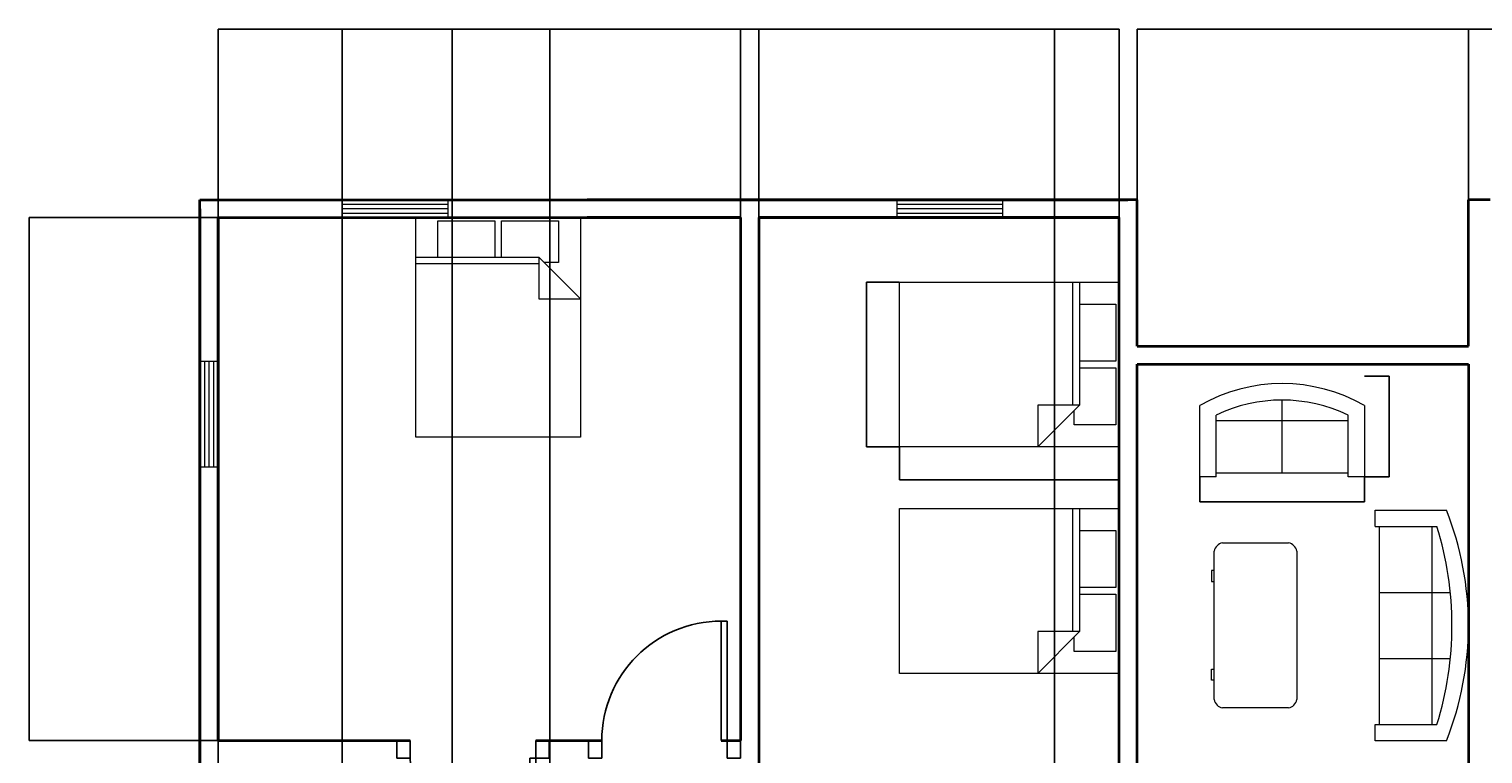
# Model space of a CAD drawing. Units: millimetres. Extents: x 31 to 27050, y -916 to 32407.
# Tile 6 of 7: x 31 to 13474, y 25704 to 32407. Entities that reach past the tile are written whole.
import ezdxf

# ---------------------------------------------------------------- set-up
doc = ezdxf.new("R2010")
doc.units = ezdxf.units.MM
for name, color, linetype, lineweight in [('A-ANNO-DIMS', 2, 'Continuous', 18), ('A-DOOR', 3, 'Continuous', 25), ('A-FURN', 8, 'Continuous', 13), ('A-GLAZ', 4, 'Continuous', 18), ('A-WALL', 7, 'Continuous', 35)]:
    doc.layers.add(name, color=color, linetype=linetype, lineweight=lineweight)
doc.styles.get("Standard").update_dxf_attribs({"font": 'arial.ttf'})
doc.dimstyles.get("Standard").update_dxf_attribs({"dimtxt": 0.18, "dimasz": 0.18, "dimexe": 0.18, "dimexo": 0.0625, "dimgap": 0.09, "dimtad": 0, "dimtih": 1, "dimtoh": 1, "dimdec": 4, "dimzin": 0, "dimdsep": 46, "dimtxsty": 'Standard', "dimcen": 0.09, "dimadec": 0, "dimazin": 0, "dimtfac": 1, "dimtdec": 4, "dimtofl": 0, "dimtmove": 0, "dimatfit": 3, "dimfxl": 1, "dimtolj": 1, "dimtzin": 0, "dimarcsym": 0})

# ---------------------------------------------------------------- blocks, each defined once
blk = doc.blocks.new('Sofa - Roundback 7 ft.')
for p, q in [((-12.00002, -32.44210000000393), (-12.00003, -6.597100000003898)), ((11.99996999999999, -32.44210000000393), (11.99997999999999, -6.597100000003898)), ((-36.000027, -34.00000000000395), (-36.000027, -11.46960000000396)), ((-35.999844, -13.38190000000397), (35.99979999999999, -13.38190000000397)), ((35.99997999999999, -34.00000000000395), (35.99997999999999, -11.46960000000396)), ((-36.000027, -32.44210000000393), (35.99997999999999, -32.44210000000393))]:
    blk.add_line(p, q)
for points in [[(-36.000027, -34.00000000000395), (-42.000027, -34.00000000000395), (-42.000027, -8.000000000003944)], [(41.99997999999999, -8.000000000003944), (41.99997999999999, -34.00000000000395), (35.99997999999999, -34.00000000000395)]]:
    blk.add_lwpolyline(points)
for centre, radius, start, end in [((0, -114.2500000000039), 114.2500000000039, 68.43141000000072, 111.5686000000006), ((-1.00000000032e-05, -127.1968000000039), 121.1967999999973, 72.72032999999948, 107.2797000000005)]:
    blk.add_arc(centre, radius, start, end)
blk = doc.blocks.new('Sofa - Roundback Loveseat 5 ft.')
for p, q in [((0, -32.44198000000246), (0, -5.999980000002448)), ((-23.99999999999999, -33.99998000000245), (-23.99999999999999, -11.46958000000243)), ((-23.99979999999998, -13.38178000000245), (23.99986, -13.38178000000245)), ((24.00004000000001, -33.99998000000245), (24.00004000000001, -11.46958000000243)), ((-23.99999999999999, -32.44198000000246), (24.00004000000001, -32.44198000000246))]:
    blk.add_line(p, q)
for points in [[(-23.99999999999999, -33.99998000000245), (-29.99999999999999, -33.99998000000245), (-29.99999999999999, -7.999980000002448)], [(30.00004000000001, -7.999980000002448), (30.00004000000001, -33.99998000000245), (24.00004000000001, -33.99998000000245)]]:
    blk.add_lwpolyline(points)
for centre, radius, start, end in [((0, -60.24998000000245), 60.24998000000245, 60.13715000000122, 119.862800000004), ((0, -61.38438000000245), 55.38444000000723, 64.32083000000306, 115.6791999999996)]:
    blk.add_arc(centre, radius, start, end)
blk = doc.blocks.new('Desk - 30 x 60 in.')
for p, q in [((-26.999995, 0), (26.999995, 0)), ((-29.999995, -27), (-29.999995, -3)), ((29.999995, -3), (29.999995, -27)), ((26.999995, -30), (-26.999995, -30)), ((-20.000005, -30), (-20.000005, -31)), ((-20.000005, -31), (-16.000005, -31)), ((-16.000005, -31), (-16.000005, -30)), ((15.999995, -31), (15.999995, -30)), ((19.999995, -31), (15.999995, -31)), ((19.999995, -30), (19.999995, -31))]:
    blk.add_line(p, q)
for centre, radius, start, end in [((-26.499995, -3.5), 3.535534000004229, 98.1300999999916, 171.8698999999352), ((26.499995, -3.5), 3.535533999997753, 8.130102000022115, 81.8698999999439), ((-26.499995, -26.5), 3.535534000000845, 188.1301000000653, 261.8699000000085), ((26.499995, -26.5), 3.535534000004826, 278.1301000000561, 351.8698999999439)]:
    blk.add_arc(centre, radius, start, end)
blk = doc.blocks.new('Bed - Queen')
for p, q in [((0, -80.00003000000002), (0, 0)), ((0, 0), (59.99998999999999, 0)), ((59.99998999999999, 0), (59.99998999999999, -80.00003000000002)), ((7.99999, -1.200000000000017), (28.79998, -1.200000000000017)), ((7.99999, -14.4), (7.99999, -1.200000000000017)), ((28.79998, -1.200000000000017), (28.79998, -14.4)), ((31.19999, -1.200000000000017), (51.99999000000001, -1.200000000000017)), ((31.19999, -14.4), (31.19999, -1.200000000000017)), ((51.99999000000001, -1.200000000000017), (51.99999000000001, -16.4)), ((0, -14.4), (44.79999999999999, -14.4)), ((59.99998999999999, -29.60000000000001), (44.79999999999999, -14.4)), ((44.79999999999999, -14.4), (44.79999999999999, -29.60000000000001)), ((44.79999999999999, -16.80000000000001), (0, -16.80000000000001)), ((51.99999000000001, -16.4), (46.79936, -16.4)), ((44.79999999999999, -29.60000000000001), (59.99998999999999, -29.60000000000001)), ((59.99998999999999, -80.00003000000002), (0, -80.00003000000002))]:
    blk.add_line(p, q)
blk = doc.blocks.new('Window - Wood Frame 36 in. Wide plan')
for p, q in [((0, 6), (0, 0)), ((36, 6), (36, 0)), ((0, 4.5), (36, 4.5)), ((0, 3), (36, 3)), ((0, 1.5), (36, 1.5))]:
    blk.add_line(p, q)
blk = doc.blocks.new('DOOR-SINGLE-1104')
for p, q in [((56.41678681898429, 1104.337341461596), (-7.18501e-11, 1104.337341461596)), ((-7.18501e-11, 1104.337341461596), (-7.18501e-11, 3.638e-12)), ((56.41678681898429, 7.276e-12), (56.41678681898429, 1104.337341461596)), ((-1226.913698425656, -163.8831223050438), (-1226.913698425656, 3.638e-12)), ((-1104.337341461589, 3.638e-12), (-1226.913698425656, 7.276e-12)), ((-1104.337341461589, 3.638e-12), (-1104.337341461589, -163.8831223050438)), ((-7.18501e-11, 3.638e-12), (56.41678681898429, 7.276e-12)), ((56.41678681898429, -163.8831223050438), (56.41678681898429, 3.638e-12)), ((56.41678681898429, 3.638e-12), (178.9931437830519, 3.638e-12)), ((178.9931437830519, 3.638e-12), (178.9931437830519, -163.8831223050438)), ((-1104.337341461589, -163.8831223050438), (-1226.913698425656, -163.8831223050438)), ((178.9931437830519, -163.8831223050438), (56.41678681898429, -163.8831223050438))]:
    blk.add_line(p, q)
blk.add_arc((0, 3.638e-12), 1104.337341461589, 90, 180)
blk = doc.blocks.new('*D18')
at = {"layer": 'A-ANNO-DIMS', "color": 0, "lineweight": -2, "transparency": 16777216}
for p, q in [((8078.02123511446, 28542.79574648087), (8078.02123511446, 28237.87813218087)), ((10110.02199711446, 28542.79574648087), (10110.02199711446, 28237.87813218087)), ((8078.201235114461, 28238.05813218087), (9092.578362362754, 28238.05813218087)), ((10109.84199711446, 28238.05813218087), (9095.464869866166, 28238.05813218087))]:
    blk.add_line(p, q, dxfattribs=at)
at = {"layer": 'A-ANNO-DIMS', "color": 0, "transparency": 16777216}
for points in [[(8078.201235114461, 28238.08813218087), (8078.201235114461, 28238.02813218087), (8078.02123511446, 28238.05813218087)], [(10109.84199711446, 28238.08813218087), (10109.84199711446, 28238.02813218087), (10110.02199711446, 28238.05813218087)]]:
    blk.add_solid(points, dxfattribs=at)
at = {"layer": 'Defpoints', "color": 0, "transparency": 16777216}
for p in [(8078.02123511446, 28542.85824648087), (10110.02199711446, 28542.85824648087), (10110.02199711446, 28238.05813218087)]:
    blk.add_point(p, dxfattribs=at)
at = {"layer": 'A-ANNO-DIMS', "color": 0, "transparency": 16777216, "insert": (9094.02161611446, 28238.05813218087), "char_height": 0.18, "attachment_point": 5}
blk.add_mtext('\\A1;QUEEN BED 2032 TYP.', dxfattribs=at)
blk = doc.blocks.new('*D19')
at = {"layer": 'A-ANNO-DIMS', "color": 0, "lineweight": -2, "transparency": 16777216}
for p, q in [((8077.958735114462, 30066.85799248089), (7773.041120814466, 30066.85799248089)), ((7773.221120814466, 30066.67799248088), (7773.221120814466, 29305.04002261868)), ((7773.221120814466, 28543.03824648089), (7773.221120814466, 29304.6762163431)), ((8077.958735114462, 28542.85824648089), (7773.041120814466, 28542.85824648089))]:
    blk.add_line(p, q, dxfattribs=at)
at = {"layer": 'A-ANNO-DIMS', "color": 0, "transparency": 16777216}
for points in [[(7773.191120814466, 30066.67799248088), (7773.251120814466, 30066.67799248088), (7773.221120814466, 30066.85799248089)], [(7773.191120814466, 28543.03824648089), (7773.251120814466, 28543.03824648089), (7773.221120814466, 28542.85824648089)]]:
    blk.add_solid(points, dxfattribs=at)
at = {"layer": 'Defpoints', "color": 0, "transparency": 16777216}
for p in [(8078.021235114462, 30066.85799248089), (7773.221120814466, 28542.85824648089), (8078.021235114462, 28542.85824648089)]:
    blk.add_point(p, dxfattribs=at)
at = {"layer": 'A-ANNO-DIMS', "color": 0, "transparency": 16777216, "insert": (7773.221120814473, 29304.85811948088), "char_height": 0.18, "attachment_point": 5}
blk.add_mtext('\\A1;1524 TYP.', dxfattribs=at)
blk = doc.blocks.new('*D36')
at = {"layer": 'A-ANNO-DIMS', "color": 0, "lineweight": -2, "transparency": 16777216}
for p, q in [((10855.59232014758, 28264.73272793006), (10855.59232014758, 28036.01507553007)), ((12379.59333614758, 28264.73272793006), (12379.59333614758, 28036.01507553007)), ((10855.77232014758, 28036.19507553007), (11616.23012009846, 28036.19507553007)), ((12379.41333614758, 28036.19507553007), (11618.95553619669, 28036.19507553007))]:
    blk.add_line(p, q, dxfattribs=at)
at = {"layer": 'A-ANNO-DIMS', "color": 0, "transparency": 16777216}
for points in [[(10855.77232014758, 28036.22507553006), (10855.77232014758, 28036.16507553007), (10855.59232014758, 28036.19507553007)], [(12379.41333614758, 28036.22507553006), (12379.41333614758, 28036.16507553007), (12379.59333614758, 28036.19507553007)]]:
    blk.add_solid(points, dxfattribs=at)
at = {"layer": 'Defpoints', "color": 0, "transparency": 16777216}
for p in [(10855.59232014758, 28264.79522793006), (12379.59333614758, 28264.79522793006), (12379.59333614758, 28036.19507553007)]:
    blk.add_point(p, dxfattribs=at)
at = {"layer": 'A-ANNO-DIMS', "color": 0, "transparency": 16777216, "insert": (11617.59282814758, 28036.19507553007), "char_height": 0.18, "attachment_point": 5}
blk.add_mtext('\\A1;LOVESEAT 1524 TYP.', dxfattribs=at)
blk = doc.blocks.new('*D37')
at = {"layer": 'A-ANNO-DIMS', "color": 0, "lineweight": -2, "transparency": 16777216}
for p, q in [((12379.65583614758, 29196.12811589219), (12608.37348854759, 29196.12811589219)), ((12608.19348854759, 29195.94811589218), (12608.19348854759, 28730.64363644047)), ((12608.19348854759, 28264.97522793008), (12608.19348854759, 28730.2797073818)), ((12379.65583614758, 28264.79522793008), (12608.37348854759, 28264.79522793008))]:
    blk.add_line(p, q, dxfattribs=at)
at = {"layer": 'A-ANNO-DIMS', "color": 0, "transparency": 16777216}
for points in [[(12608.16348854759, 29195.94811589218), (12608.22348854759, 29195.94811589218), (12608.19348854759, 29196.12811589219)], [(12608.16348854759, 28264.97522793008), (12608.2234885476, 28264.97522793008), (12608.19348854759, 28264.79522793008)]]:
    blk.add_solid(points, dxfattribs=at)
at = {"layer": 'Defpoints', "color": 0, "transparency": 16777216}
for p in [(12379.59333614758, 29196.12811589219), (12608.19348854759, 29196.12811589219), (12379.59333614758, 28264.79522793008)]:
    blk.add_point(p, dxfattribs=at)
at = {"layer": 'A-ANNO-DIMS', "color": 0, "transparency": 16777216, "insert": (12608.1934885476, 28730.46167191112), "char_height": 0.18, "attachment_point": 5}
blk.add_mtext('\\A1;931 TYP.', dxfattribs=at)
blk = doc.blocks.new('*D48')
at = {"layer": 'A-ANNO-DIMS', "color": 0, "lineweight": -2, "transparency": 16777216}
for p, q in [((1778.372648, 30663.710636), (1778.372648, 32406.711259)), ((1778.552648, 32406.531259), (4193.835849103002, 32406.531259)), ((6609.841997, 32406.531259), (4194.558795896999, 32406.531259)), ((6610.021997, 30663.710636), (6610.021997, 32406.711259))]:
    blk.add_line(p, q, dxfattribs=at)
at = {"layer": 'A-ANNO-DIMS', "color": 0, "transparency": 16777216}
for points in [[(1778.552648, 32406.561259), (1778.552648, 32406.501259), (1778.372648, 32406.531259)], [(6609.841997, 32406.561259), (6609.841997, 32406.501259), (6610.021997, 32406.531259)]]:
    blk.add_solid(points, dxfattribs=at)
at = {"layer": 'Defpoints', "color": 0, "transparency": 16777216}
for p in [(6610.021997, 32406.531259), (1778.372648, 30663.648136), (6610.021997, 30663.648136)]:
    blk.add_point(p, dxfattribs=at)
at = {"layer": 'A-ANNO-DIMS', "color": 0, "transparency": 16777216, "insert": (4194.1973225, 32406.531259), "char_height": 0.18, "attachment_point": 5}
blk.add_mtext('\\A1;4832', dxfattribs=at)
blk = doc.blocks.new('*D49')
at = {"layer": 'A-ANNO-DIMS', "color": 0, "lineweight": -2, "transparency": 16777216}
for p, q in [((6778.372648, 30663.710636), (6778.372648, 32406.711259)), ((6778.552648, 32406.531259), (8443.733816360846, 32406.531259)), ((10109.841997, 32406.531259), (8444.660828639157, 32406.531259)), ((10110.021997, 30663.710636), (10110.021997, 32406.711259))]:
    blk.add_line(p, q, dxfattribs=at)
at = {"layer": 'A-ANNO-DIMS', "color": 0, "transparency": 16777216}
for points in [[(6778.552648, 32406.561259), (6778.552648, 32406.501259), (6778.372648, 32406.531259)], [(10109.841997, 32406.561259), (10109.841997, 32406.501259), (10110.021997, 32406.531259)]]:
    blk.add_solid(points, dxfattribs=at)
at = {"layer": 'Defpoints', "color": 0, "transparency": 16777216}
for p in [(10110.021997, 32406.531259), (6778.372648, 30663.648136), (10110.021997, 30663.648136)]:
    blk.add_point(p, dxfattribs=at)
at = {"layer": 'A-ANNO-DIMS', "color": 0, "transparency": 16777216, "insert": (8444.1973225, 32406.531259), "char_height": 0.18, "attachment_point": 5}
blk.add_mtext('\\A1;3331.6', dxfattribs=at)
blk = doc.blocks.new('*D50')
at = {"layer": 'A-ANNO-DIMS', "color": 0, "lineweight": -2, "transparency": 16777216}
for p, q in [((10278.372648, 30827.593759), (10278.372648, 32406.711259)), ((10278.552648, 32406.531259), (11809.1212005955, 32406.531259)), ((13340.405333, 32406.531259), (11809.8367804045, 32406.531259)), ((13340.585333, 30827.593759), (13340.585333, 32406.711259))]:
    blk.add_line(p, q, dxfattribs=at)
at = {"layer": 'A-ANNO-DIMS', "color": 0, "transparency": 16777216}
for points in [[(10278.552648, 32406.561259), (10278.552648, 32406.501259), (10278.372648, 32406.531259)], [(13340.405333, 32406.561259), (13340.405333, 32406.501259), (13340.585333, 32406.531259)]]:
    blk.add_solid(points, dxfattribs=at)
at = {"layer": 'Defpoints', "color": 0, "transparency": 16777216}
for p in [(13340.585333, 32406.531259), (10278.372648, 30827.531259), (13340.585333, 30827.531259)]:
    blk.add_point(p, dxfattribs=at)
at = {"layer": 'A-ANNO-DIMS', "color": 0, "transparency": 16777216, "insert": (11809.4789905, 32406.531259), "char_height": 0.18, "attachment_point": 5}
blk.add_mtext('\\A1;3062', dxfattribs=at)
blk = doc.blocks.new('*D51')
at = {"layer": 'A-ANNO-DIMS', "color": 0, "lineweight": -2, "transparency": 16777216}
for p, q in [((13340.585333, 30827.593759), (13340.585333, 32406.711259)), ((13340.765333, 32406.531259), (13540.29317065348, 32406.531259)), ((13740.405333, 32406.531259), (13540.87749534652, 32406.531259)), ((13740.585333, 30827.593759), (13740.585333, 32406.711259))]:
    blk.add_line(p, q, dxfattribs=at)
at = {"layer": 'A-ANNO-DIMS', "color": 0, "transparency": 16777216}
for points in [[(13340.765333, 32406.561259), (13340.765333, 32406.501259), (13340.585333, 32406.531259)], [(13740.405333, 32406.561259), (13740.405333, 32406.501259), (13740.585333, 32406.531259)]]:
    blk.add_solid(points, dxfattribs=at)
at = {"layer": 'Defpoints', "color": 0, "transparency": 16777216}
for p in [(13740.585333, 32406.531259), (13340.585333, 30827.531259), (13740.585333, 30827.531259)]:
    blk.add_point(p, dxfattribs=at)
at = {"layer": 'A-ANNO-DIMS', "color": 0, "transparency": 16777216, "insert": (13540.585333, 32406.531259), "char_height": 0.18, "attachment_point": 5}
blk.add_mtext('\\A1;400', dxfattribs=at)
blk = doc.blocks.new('*D52')
at = {"layer": 'A-ANNO-DIMS', "color": 0, "lineweight": -2, "transparency": 16777216}
for p, q in [((1778.310148000001, 30663.64813600002), (30.84199699999933, 30663.64813600002)), ((31.02199699999949, 30663.46813600001), (31.02199700000003, 28245.77166202935)), ((31.02199700000057, 25827.71125900002), (31.02199700000003, 28245.40773297068)), ((1778.310148000001, 25827.53125900001), (30.8419970000004, 25827.53125900001))]:
    blk.add_line(p, q, dxfattribs=at)
at = {"layer": 'A-ANNO-DIMS', "color": 0, "transparency": 16777216}
for points in [[(30.99199699999949, 30663.46813600001), (31.05199699999949, 30663.46813600001), (31.02199699999949, 30663.64813600002)], [(30.99199700000057, 25827.71125900002), (31.05199700000057, 25827.71125900002), (31.02199700000057, 25827.53125900001)]]:
    blk.add_solid(points, dxfattribs=at)
at = {"layer": 'Defpoints', "color": 0, "transparency": 16777216}
for p in [(31.02199699999949, 30663.64813600002), (1778.372648000001, 30663.64813600002), (1778.372648000001, 25827.53125900001)]:
    blk.add_point(p, dxfattribs=at)
at = {"layer": 'A-ANNO-DIMS', "color": 0, "transparency": 16777216, "insert": (31.02199700000802, 28245.58969750001), "char_height": 0.18, "attachment_point": 5}
blk.add_mtext('\\A1;4836', dxfattribs=at)
blk = doc.blocks.new('*D61')
at = {"layer": 'A-ANNO-DIMS', "color": 0, "lineweight": -2, "transparency": 16777216}
for p, q in [((1778.372648, 7250.606205), (1778.372648000001, 32406.711259)), ((1778.552648000001, 32406.531259), (3312.109331318556, 32406.531259)), ((4846.592413000001, 32406.531259), (3313.035729681448, 32406.531259)), ((4846.772413, 7250.606205), (4846.772413000001, 32406.711259))]:
    blk.add_line(p, q, dxfattribs=at)
at = {"layer": 'A-ANNO-DIMS', "color": 0, "transparency": 16777216}
for points in [[(1778.552648000001, 32406.561259), (1778.552648000001, 32406.501259), (1778.372648000001, 32406.531259)], [(4846.592413000001, 32406.561259), (4846.592413000001, 32406.501259), (4846.772413000001, 32406.531259)]]:
    blk.add_solid(points, dxfattribs=at)
at = {"layer": 'Defpoints', "color": 0, "transparency": 16777216}
for p in [(4846.772413000001, 32406.531259), (1778.372648, 7250.543705), (4846.772413, 7250.543705)]:
    blk.add_point(p, dxfattribs=at)
at = {"layer": 'A-ANNO-DIMS', "color": 0, "transparency": 16777216, "insert": (3312.572530500002, 32406.531259), "char_height": 0.18, "attachment_point": 5}
blk.add_mtext('\\A1;3068.4', dxfattribs=at)
blk = doc.blocks.new('*D66')
at = {"layer": 'A-ANNO-DIMS', "color": 0, "lineweight": -2, "transparency": 16777216}
for p, q in [((2925.691486, 19025.498224), (2925.691486000001, 32406.711259)), ((2925.871486000001, 32406.531259), (6219.151999023875, 32406.531259)), ((9513.151407, 32406.531259), (6219.870893976127, 32406.531259)), ((9513.331407, 19025.498224), (9513.331407, 32406.711259))]:
    blk.add_line(p, q, dxfattribs=at)
at = {"layer": 'A-ANNO-DIMS', "color": 0, "transparency": 16777216}
for points in [[(2925.871486000001, 32406.561259), (2925.871486000001, 32406.501259), (2925.691486000001, 32406.531259)], [(9513.151407, 32406.561259), (9513.151407, 32406.501259), (9513.331407, 32406.531259)]]:
    blk.add_solid(points, dxfattribs=at)
at = {"layer": 'Defpoints', "color": 0, "transparency": 16777216}
for p in [(9513.331407, 32406.531259), (2925.691486, 19025.435724), (9513.331407, 19025.435724)]:
    blk.add_point(p, dxfattribs=at)
at = {"layer": 'A-ANNO-DIMS', "color": 0, "transparency": 16777216, "insert": (6219.511446500001, 32406.531259), "char_height": 0.18, "attachment_point": 5}
blk.add_mtext('\\A1;6588', dxfattribs=at)
blk = doc.blocks.new('*D89')
at = {"layer": 'A-ANNO-DIMS', "color": 0, "lineweight": -2, "transparency": 16777216}
for p, q in [((6610.021997, 30663.710636), (6610.021997, 32406.711259)), ((6610.201997, 32406.531259), (6693.741490303548, 32406.531259)), ((6778.192648, 32406.531259), (6694.653154696453, 32406.531259)), ((6778.372648, 30663.710636), (6778.372648, 32406.711259))]:
    blk.add_line(p, q, dxfattribs=at)
at = {"layer": 'A-ANNO-DIMS', "color": 0, "transparency": 16777216}
for points in [[(6610.201997, 32406.561259), (6610.201997, 32406.501259), (6610.021997, 32406.531259)], [(6778.192648, 32406.561259), (6778.192648, 32406.501259), (6778.372648, 32406.531259)]]:
    blk.add_solid(points, dxfattribs=at)
at = {"layer": 'Defpoints', "color": 0, "transparency": 16777216}
for p in [(6778.372648, 32406.531259), (6610.021997, 30663.648136), (6778.372648, 30663.648136)]:
    blk.add_point(p, dxfattribs=at)
at = {"layer": 'A-ANNO-DIMS', "color": 0, "transparency": 16777216, "insert": (6694.197322499999, 32406.531259), "char_height": 0.18, "attachment_point": 5}
blk.add_mtext('\\A1;168.35', dxfattribs=at)
blk = doc.blocks.new('*D94')
at = {"layer": 'A-ANNO-DIMS', "color": 0, "lineweight": -2, "transparency": 16777216}
for p, q in [((2925.691486, 16977.007419), (2925.691486000001, 32406.711259)), ((2925.871486000001, 32406.531259), (3434.121002435881, 32406.531259)), ((3943.281201000001, 32406.531259), (3435.031684564121, 32406.531259)), ((3943.461201, 17070.178763), (3943.461201000001, 32406.711259))]:
    blk.add_line(p, q, dxfattribs=at)
at = {"layer": 'A-ANNO-DIMS', "color": 0, "transparency": 16777216}
for points in [[(2925.871486000001, 32406.561259), (2925.871486000001, 32406.501259), (2925.691486000001, 32406.531259)], [(3943.281201000001, 32406.561259), (3943.281201000001, 32406.501259), (3943.461201000001, 32406.531259)]]:
    blk.add_solid(points, dxfattribs=at)
at = {"layer": 'Defpoints', "color": 0, "transparency": 16777216}
for p in [(3943.461201000001, 32406.531259), (2925.691486, 16976.944919), (3943.461201, 17070.116263)]:
    blk.add_point(p, dxfattribs=at)
at = {"layer": 'A-ANNO-DIMS', "color": 0, "transparency": 16777216, "insert": (3434.576343500001, 32406.531259), "char_height": 0.18, "attachment_point": 5}
blk.add_mtext('\\A1;1017.8', dxfattribs=at)

msp = doc.modelspace()

# ---------------------------------------------------------------- linework, layer by layer
at = {"layer": 'A-DOOR'}
for p, q in [((6487.445640150399, 26931.86860013333), (6487.445640150399, 26931.86860013333)), ((6610.021997114467, 25827.53125867173), (6487.445640150399, 25827.53125867174))]:
    msp.add_line(p, q, dxfattribs=at)
at = {"layer": 'A-WALL'}
for p, q in [((1610.021997114467, 30744.38037777559), (1610.021997114467, 30827.53125867173)), ((1610.021997114467, 30827.53125867173), (1728.177251255896, 30827.53125867173)), ((1690.585332610448, 30827.53125867173), (10190.58533261045, 30827.53125867173)), ((10278.37264782516, 30827.53125867173), (5190.585332610459, 30827.53125867173)), ((10278.37264782516, 30663.64813636668), (10278.37264782516, 30827.53125867173)), ((13540.58533261045, 30827.53125867174), (13340.58533261045, 30827.53125867174)), ((13340.58533261045, 30744.3803777756), (13340.58533261045, 30827.53125867173)), ((1610.021997114467, 30744.38037777559), (1610.021997114467, 19106.16796530105)), ((1610.021997114467, 30744.38037777559), (1610.021997114467, 25744.38037777559)), ((1610.021997114469, 19025.43572389214), (1610.021997114469, 30744.3803777756)), ((1778.372647825163, 30663.64813636668), (6610.021997114468, 30663.64813636668)), ((1778.372647825161, 30663.64813636668), (1778.372647825161, 25827.53125867173)), ((1778.372647825161, 30663.64813636668), (1778.372647825161, 25827.53125867174)), ((1778.372647825163, 25827.53125867173), (1778.372647825163, 30663.64813636667)), ((6610.021997114467, 30663.64813636668), (5190.585332610459, 30663.64813636668)), ((6610.021997114468, 30663.64813636669), (6610.021997114468, 25827.53125867174)), ((6778.372647825161, 30663.64813636668), (6778.372647825161, 25282.64192458121)), ((10110.02199711446, 30663.64813636668), (6778.372647825162, 30663.64813636668)), ((6778.372647825162, 30663.64813636669), (10110.02199711446, 30663.64813636669)), ((10110.02199711446, 25282.64192458121), (10110.02199711446, 30663.64813636668)), ((10278.37264782516, 29473.25786145121), (10278.37264782516, 30663.64813636668)), ((13340.58533261045, 29473.25786145121), (13340.58533261045, 30744.3803777756)), ((10278.37264782516, 29473.25786145121), (13340.58533261045, 29473.25786145121)), ((10278.37264782516, 29309.37473914616), (13340.58533261045, 29309.37473914617)), ((10278.37264782516, 24473.25786145121), (10278.37264782516, 29309.37473914616)), ((13340.58533261045, 29309.37473914617), (13340.58533261045, 24473.25786145121)), ((1778.372647825163, 25827.53125867173), (3555.45629841193, 25827.53125867174)), ((4716.210426692502, 25827.53125867174), (5326.691511869826, 25827.53125867173)), ((6431.028853331344, 25827.53125867174), (6610.021997114467, 25827.53125867173))]:
    msp.add_line(p, q, dxfattribs=at)

# ---------------------------------------------------------------- block references
at = {"layer": 'A-DOOR'}
msp.add_blockref('DOOR-SINGLE-1104', (6431.028853331415, 25827.53125867173), dxfattribs=at)
at = {"layer": 'A-DOOR', "extrusion": (0, 0, -1), "zscale": -1, "rotation": 180}
msp.add_blockref('DOOR-SINGLE-1104', (-4659.793639873515, 25663.6481363667), dxfattribs=at)
at = {"layer": 'A-FURN', "xscale": 25.4, "yscale": 25.4, "zscale": 25.4}
for name, p in [('Bed - Queen', (3606.233526750235, 30663.64813636668)), ('Sofa - Roundback Loveseat 5 ft.', (11617.59232014758, 29128.39471993013))]:
    msp.add_blockref(name, p, dxfattribs=at)
at = {"layer": 'A-FURN', "xscale": 25.4, "yscale": 25.4, "zscale": 25.4, "rotation": 270}
for name, p in [('Bed - Queen', (10110.02199711446, 30066.85799248087)), ('Bed - Queen', (10110.02199711446, 27973.14503047395)), ('Sofa - Roundback 7 ft.', (13340.58533261045, 26891.31630029868)), ('Desk - 30 x 60 in.', (11752.38827730674, 26892.70491289827))]:
    msp.add_blockref(name, p, dxfattribs=at)
at = {"layer": 'A-GLAZ', "xscale": 27.11229900122799, "yscale": 27.11229900122799, "zscale": 27.11229900122799}
for p in [(2925.548195503419, 30664.85746466437), (8055.413904695946, 30664.85746466437)]:
    msp.add_blockref('Window - Wood Frame 36 in. Wide plan', p, dxfattribs=at)
at = {"layer": 'A-GLAZ', "xscale": 27.11229900122799, "yscale": 27.11229900122799, "zscale": 27.11229900122799, "rotation": 90}
msp.add_blockref('Window - Wood Frame 36 in. Wide plan', (1778.372647825162, 28358.69751835588), dxfattribs=at)

# ---------------------------------------------------------------- dimensions: what is measured, and where the dimension line sits
at = {"layer": 'A-ANNO-DIMS'}
for base, p1, p2, override, picture, middle in [((6610.021997, 32406.531259), (1778.372648, 30663.648136), (6610.021997, 30663.648136), {"dimdec": 0, "dimlfac": 1, "dimrnd": 0, "dimzin": 0, "dimdsep": 46, "dimlunit": 2}, '*D48', (4194.1973225, 32406.531259)), ((4846.772413000001, 32406.531259), (1778.372648, 7250.543705), (4846.772413, 7250.543705), {"dimdec": 1, "dimlfac": 1, "dimrnd": 0, "dimzin": 0, "dimdsep": 46, "dimlunit": 2}, '*D61', (3312.572530500002, 32406.531259)), ((9513.331407, 32406.531259), (2925.691486, 19025.435724), (9513.331407, 19025.435724), {"dimdec": 0, "dimlfac": 1, "dimrnd": 0, "dimzin": 0, "dimdsep": 46, "dimlunit": 2}, '*D66', (6219.511446500001, 32406.531259)), ((3943.461201000001, 32406.531259), (2925.691486, 16976.944919), (3943.461201, 17070.116263), {"dimdec": 1, "dimlfac": 1, "dimrnd": 0, "dimzin": 0, "dimdsep": 46, "dimlunit": 2}, '*D94', (3434.576343500001, 32406.531259)), ((6778.372648, 32406.531259), (6610.021997, 30663.648136), (6778.372648, 30663.648136), {"dimdec": 2, "dimlfac": 1, "dimrnd": 0, "dimzin": 0, "dimdsep": 46, "dimlunit": 2}, '*D89', (6694.197322499999, 32406.531259)), ((10110.021997, 32406.531259), (6778.372648, 30663.648136), (10110.021997, 30663.648136), {"dimdec": 1, "dimlfac": 1, "dimrnd": 0, "dimzin": 0, "dimdsep": 46, "dimlunit": 2}, '*D49', (8444.1973225, 32406.531259)), ((13340.585333, 32406.531259), (10278.372648, 30827.531259), (13340.585333, 30827.531259), {"dimdec": 0, "dimlfac": 1, "dimrnd": 0, "dimzin": 0, "dimdsep": 46, "dimlunit": 2}, '*D50', (11809.4789905, 32406.531259)), ((13740.585333, 32406.531259), (13340.585333, 30827.531259), (13740.585333, 30827.531259), {"dimdec": 0, "dimlfac": 1, "dimrnd": 0, "dimzin": 0, "dimdsep": 46, "dimlunit": 2}, '*D51', (13540.585333, 32406.531259))]:
    dim = msp.add_linear_dim(base=base, p1=p1, p2=p2, dimstyle='Standard', override=override, dxfattribs=at)
    dim.commit()
    dim.dimension.update_dxf_attribs({"geometry": picture, "text_midpoint": middle})
dim = msp.add_linear_dim(base=(31.02199699999949, 30663.64813600002), p1=(1778.372648, 25827.531259), p2=(1778.372648, 30663.648136), angle=90, dimstyle='Standard', override={"dimdec": 0, "dimlfac": 1, "dimrnd": 0, "dimzin": 0, "dimdsep": 46, "dimlunit": 2}, dxfattribs=at)
dim.commit()
dim.dimension.update_dxf_attribs({"geometry": '*D52', "text_midpoint": (31.02199700000802, 28245.58969750001)})
for base, p1, p2, angle, picture, middle in [((7773.221120814466, 28542.85824648089), (8078.02123511446, 30066.85799248087), (8078.02123511446, 28542.85824648087), 270, '*D19', (7773.221120814473, 29304.85811948088)), ((12608.19348854759, 29196.12811589219), (12379.59333614758, 28264.79522793006), (12379.59333614758, 29196.12811589217), 90, '*D37', (12608.1934885476, 28730.46167191112))]:
    dim = msp.add_linear_dim(base=base, p1=p1, p2=p2, angle=angle, text='<> TYP.', dimstyle='Standard', override={"dimdec": 0, "dimlfac": 1, "dimrnd": 0, "dimzin": 0, "dimdsep": 46, "dimlunit": 2}, dxfattribs=at)
    dim.commit()
    dim.dimension.update_dxf_attribs({"geometry": picture, "text_midpoint": middle})
for base, p1, p2, text, picture, middle in [((10110.02199711446, 28238.05813218087), (8078.02123511446, 28542.85824648087), (10110.02199711446, 28542.85824648087), 'QUEEN BED <> TYP.', '*D18', (9094.02161611446, 28238.05813218087)), ((12379.59333614758, 28036.19507553007), (10855.59232014758, 28264.79522793006), (12379.59333614758, 28264.79522793006), 'LOVESEAT <> TYP.', '*D36', (11617.59282814758, 28036.19507553007))]:
    dim = msp.add_linear_dim(base=base, p1=p1, p2=p2, text=text, dimstyle='Standard', override={"dimdec": 0, "dimlfac": 1, "dimrnd": 0, "dimzin": 0, "dimdsep": 46, "dimlunit": 2}, dxfattribs=at)
    dim.commit()
    dim.dimension.update_dxf_attribs({"geometry": picture, "text_midpoint": middle})

doc.saveas('drawing.dxf')
